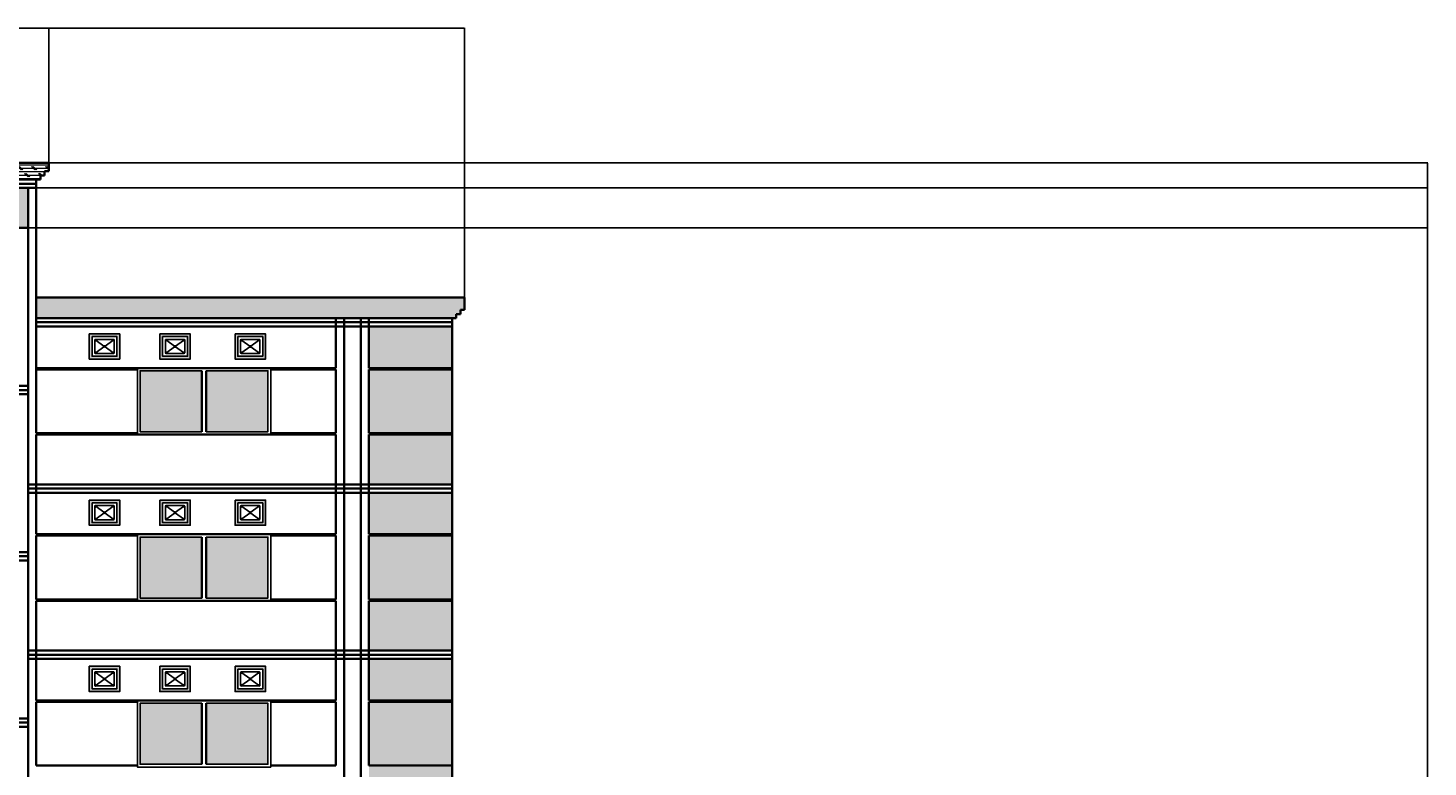
# Model space of a CAD drawing. Units: inches. Extents: x -742 to 1386, y -64 to 951.
# Tile 8 of 8: x 376 to 1386, y 418 to 951. Entities that reach past the tile are written whole.
import ezdxf

# ---------------------------------------------------------------- set-up
doc = ezdxf.new("R2010")
doc.units = ezdxf.units.IN
doc.header["$MEASUREMENT"] = 0
for name, color, linetype, lineweight in [('A-ANNO-DIMS', 2, 'Continuous', 18), ('A-ELEV', 7, 'Continuous', 35), ('A-ELEV-PATT', 252, 'Continuous', 13), ('A-GLAZ', 4, 'Continuous', 25), ('A-WALL-PATT', 8, 'Continuous', 13)]:
    doc.layers.add(name, color=color, linetype=linetype, lineweight=lineweight)
doc.styles.get("Standard").update_dxf_attribs({"font": 'arial.ttf'})
doc.dimstyles.get("Standard").update_dxf_attribs({"dimtxt": 0.18, "dimasz": 0.18, "dimexe": 0.18, "dimexo": 0.0625, "dimgap": 0.09, "dimtad": 0, "dimtih": 1, "dimtoh": 1, "dimdec": 4, "dimzin": 0, "dimdsep": 46, "dimtxsty": 'Standard', "dimcen": 0.09, "dimadec": 0, "dimazin": 0, "dimtfac": 1, "dimtdec": 4, "dimtofl": 0, "dimtmove": 0, "dimatfit": 3, "dimfxl": 1, "dimtolj": 1, "dimtzin": 0, "dimarcsym": 0})

# ---------------------------------------------------------------- blocks, each defined once
blk = doc.blocks.new('VENT-WIN')
h = blk.add_hatch(color=256)
h.dxf.hatch_style = 1
h.paths.add_polyline_path([(11.5, 9.1, 1), (10.5, 9.1, 1)])
h.paths.add_polyline_path([(16.9, 13.7, 1), (18, 13.7, 1)])
h.paths.add_polyline_path([(18, 4.5, 1), (16.9, 4.5, 1)])
h.paths.add_polyline_path([(5, 4.5, 1), (4, 4.5, 1)])
h.paths.add_polyline_path([(4, 13.7, 1), (5, 13.7, 1)])
for p, q in [((5, 13.5), (10.6, 9.4)), ((11.4, 9.4), (17, 13.5)), ((5, 4.7), (10.6, 8.8)), ((11.4, 8.8), (17, 4.7))]:
    blk.add_line(p, q)
for points in [[(0, 18.2), (22, 18.2), (22, 0), (0, 0)], [(2, 16.2), (20, 16.2), (20, 2), (2, 2)]]:
    blk.add_lwpolyline(points, close=True)
for points in [[(4, 4.5), (4, 13.7)], [(4.5, 14.2), (17.5, 14.2)], [(18, 13.7), (18, 4.5)], [(17.5, 4), (4.5, 4)]]:
    blk.add_lwpolyline(points)
for centre in [(4.5, 13.7), (17.5, 13.7), (4.5, 4.5), (11, 9.1), (17.5, 4.5)]:
    blk.add_circle(centre, 0.519)
blk = doc.blocks.new('WIN-1000-2PANE')
blk.add_lwpolyline([(0, 48), (96.2, 48), (96.2, 0), (0, 0)], close=True)
for points in [[(46.6, 2), (2, 2), (2, 46), (46.6, 46)], [(49.6, 46), (94.2, 46), (94.2, 2), (49.6, 2)]]:
    blk.add_lwpolyline(points)
blk = doc.blocks.new('*D10')
at = {"layer": 'A-ANNO-DIMS', "color": 0, "lineweight": -2, "transparency": 16777216}
for p, q in [((-46.8, 756.8), (-46.8, 951.2)), ((-46.6, 951), (321.9, 951)), ((691, 951), (322.5, 951)), ((691.2, 756.8), (691.2, 951.2))]:
    blk.add_line(p, q, dxfattribs=at)
at = {"layer": 'A-ANNO-DIMS', "color": 0, "transparency": 16777216}
for points in [[(-46.6, 951.1), (-46.6, 951), (-46.8, 951)], [(691, 951.1), (691, 951), (691.2, 951)]]:
    blk.add_solid(points, dxfattribs=at)
at = {"layer": 'Defpoints', "color": 0, "transparency": 16777216}
for p in [(691.2, 951), (-46.8, 756.7), (691.2, 756.7)]:
    blk.add_point(p, dxfattribs=at)
at = {"layer": 'A-ANNO-DIMS', "color": 0, "transparency": 16777216, "insert": (322.2, 951), "char_height": 0.18, "attachment_point": 5}
blk.add_mtext('\\A1;738', dxfattribs=at)
blk = doc.blocks.new('*D11')
at = {"layer": 'A-ANNO-DIMS', "color": 0, "lineweight": -2, "transparency": 16777216}
for p, q in [((253.2, 853.8), (253.2, 951.2)), ((253.4, 951), (321.9, 951)), ((391, 951), (322.5, 951)), ((391.2, 853.8), (391.2, 951.2))]:
    blk.add_line(p, q, dxfattribs=at)
at = {"layer": 'A-ANNO-DIMS', "color": 0, "transparency": 16777216}
for points in [[(253.4, 951.1), (253.4, 951), (253.2, 951)], [(391, 951.1), (391, 951), (391.2, 951)]]:
    blk.add_solid(points, dxfattribs=at)
at = {"layer": 'Defpoints', "color": 0, "transparency": 16777216}
for p in [(391.2, 951), (253.2, 853.8), (391.2, 853.8)]:
    blk.add_point(p, dxfattribs=at)
at = {"layer": 'A-ANNO-DIMS', "color": 0, "transparency": 16777216, "insert": (322.2, 951), "char_height": 0.18, "attachment_point": 5}
blk.add_mtext('\\A1;138', dxfattribs=at)
blk = doc.blocks.new('*D39')
at = {"layer": 'A-ANNO-DIMS', "color": 0, "lineweight": -2, "transparency": 16777216}
for p, q in [((391.3, 853.8), (1386, 853.8)), ((1385.8, 853.6), (1385.8, 479.9)), ((1385.8, 105.9), (1385.8, 479.6)), ((682.3, 105.7), (1386, 105.7))]:
    blk.add_line(p, q, dxfattribs=at)
at = {"layer": 'A-ANNO-DIMS', "color": 0, "transparency": 16777216}
for points in [[(1385.8, 853.6), (1385.9, 853.6), (1385.8, 853.8)], [(1385.8, 105.9), (1385.9, 105.9), (1385.8, 105.7)]]:
    blk.add_solid(points, dxfattribs=at)
at = {"layer": 'Defpoints', "color": 0, "transparency": 16777216}
for p in [(391.2, 853.8), (682.2, 105.7), (1385.8, 105.7)]:
    blk.add_point(p, dxfattribs=at)
at = {"layer": 'A-ANNO-DIMS', "color": 0, "transparency": 16777216, "insert": (1385.8, 479.8), "char_height": 0.18, "attachment_point": 5}
blk.add_mtext('\\A1;748', dxfattribs=at)
blk = doc.blocks.new('*D57')
at = {"layer": 'A-ANNO-DIMS', "color": 0, "lineweight": -2, "transparency": 16777216}
for p, q in [((376.3, 835.8), (1386, 835.8)), ((1385.8, 835.6), (1385.8, 821.5)), ((1385.8, 807), (1385.8, 821.1)), ((346.8, 806.9), (1386, 806.9))]:
    blk.add_line(p, q, dxfattribs=at)
at = {"layer": 'A-ANNO-DIMS', "color": 0, "transparency": 16777216}
for points in [[(1385.8, 835.6), (1385.9, 835.6), (1385.8, 835.8)], [(1385.8, 807), (1385.9, 807), (1385.8, 806.9)]]:
    blk.add_solid(points, dxfattribs=at)
at = {"layer": 'Defpoints', "color": 0, "transparency": 16777216}
for p in [(376.2, 835.8), (1385.8, 835.8), (346.7, 806.9)]:
    blk.add_point(p, dxfattribs=at)
at = {"layer": 'A-ANNO-DIMS', "color": 0, "transparency": 16777216, "insert": (1385.8, 821.3), "char_height": 0.18, "attachment_point": 5}
blk.add_mtext('\\A1;28.925', dxfattribs=at)

msp = doc.modelspace()

# ---------------------------------------------------------------- hatches: boundary and pattern name
at = {"layer": 'A-ELEV-PATT'}
h = msp.add_hatch(color=256, dxfattribs=at)
h.dxf.hatch_style = 1
h.paths.add_polyline_path([(442.4136, 730.4496), (420.4263, 730.4496), (420.4263, 712.2254), (442.4136, 712.2254)])
h.paths.add_polyline_path([(440.4136, 714.2254), (422.4263, 714.2254), (422.4263, 728.4496), (440.4136, 728.4496)], flags=16)
h.paths.add_polyline_path([(493.3109, 730.4496), (471.3236, 730.4496), (471.3236, 712.2254), (493.3109, 712.2254)])
h.paths.add_polyline_path([(491.3109, 728.4496), (491.3109, 714.2254), (473.3236, 714.2254), (473.3236, 728.4496)], flags=16)
h.paths.add_polyline_path([(547.5617, 730.4496), (525.5743, 730.4496), (525.5743, 712.2254), (547.5617, 712.2254)])
h.paths.add_polyline_path([(545.5617, 728.4496), (545.5617, 714.2254), (527.5743, 714.2254), (527.5743, 728.4496)], flags=16)
h = msp.add_hatch(color=256, dxfattribs=at)
h.dxf.hatch_style = 1
h.set_gradient(color1=(0, 255, 255), name='CURVED')
h.paths.add_polyline_path([(139.7128, 703.7399), (95.1117, 703.7399), (95.1117, 659.7399), (139.7128, 659.7399)])
h.paths.add_polyline_path([(187.3139, 703.7399), (142.7128, 703.7399), (142.7128, 659.7399), (187.3139, 659.7399)])
h.paths.add_polyline_path([(501.7423, 703.7399), (457.1413, 703.7399), (457.1413, 659.7399), (501.7423, 659.7399)])
h.paths.add_polyline_path([(549.3434, 703.7399), (504.7423, 703.7399), (504.7423, 659.7399), (549.3434, 659.7399)])
h = msp.add_hatch(color=256, dxfattribs=at)
h.dxf.hatch_style = 1
h.paths.add_polyline_path([(442.4136, 610.4496), (420.4263, 610.4496), (420.4263, 592.2254), (442.4136, 592.2254)])
h.paths.add_polyline_path([(440.4136, 594.2254), (422.4263, 594.2254), (422.4263, 608.4496), (440.4136, 608.4496)], flags=16)
h.paths.add_polyline_path([(493.3109, 610.4496), (471.3236, 610.4496), (471.3236, 592.2254), (493.3109, 592.2254)])
h.paths.add_polyline_path([(491.3109, 608.4496), (491.3109, 594.2254), (473.3236, 594.2254), (473.3236, 608.4496)], flags=16)
h.paths.add_polyline_path([(547.5617, 610.4496), (525.5743, 610.4496), (525.5743, 592.2254), (547.5617, 592.2254)])
h.paths.add_polyline_path([(545.5617, 608.4496), (545.5617, 594.2254), (527.5743, 594.2254), (527.5743, 608.4496)], flags=16)
h = msp.add_hatch(color=256, dxfattribs=at)
h.dxf.hatch_style = 1
h.set_gradient(color1=(0, 255, 255), name='CURVED')
h.paths.add_polyline_path([(139.7128, 583.7399), (95.1117, 583.7399), (95.1117, 539.7399), (139.7128, 539.7399)])
h.paths.add_polyline_path([(187.3139, 583.7399), (142.7128, 583.7399), (142.7128, 539.7399), (187.3139, 539.7399)])
h.paths.add_polyline_path([(501.7423, 583.7399), (457.1413, 583.7399), (457.1413, 539.7399), (501.7423, 539.7399)])
h.paths.add_polyline_path([(549.3434, 583.7399), (504.7423, 583.7399), (504.7423, 539.7399), (549.3434, 539.7399)])
h = msp.add_hatch(color=256, dxfattribs=at)
h.dxf.hatch_style = 1
h.paths.add_polyline_path([(442.4136, 490.4496), (420.4263, 490.4496), (420.4263, 472.2254), (442.4136, 472.2254)])
h.paths.add_polyline_path([(440.4136, 474.2254), (422.4263, 474.2254), (422.4263, 488.4496), (440.4136, 488.4496)], flags=16)
h.paths.add_polyline_path([(493.3109, 490.4496), (471.3236, 490.4496), (471.3236, 472.2254), (493.3109, 472.2254)])
h.paths.add_polyline_path([(491.3109, 488.4496), (491.3109, 474.2254), (473.3236, 474.2254), (473.3236, 488.4496)], flags=16)
h.paths.add_polyline_path([(547.5617, 490.4496), (525.5743, 490.4496), (525.5743, 472.2254), (547.5617, 472.2254)])
h.paths.add_polyline_path([(545.5617, 488.4496), (545.5617, 474.2254), (527.5743, 474.2254), (527.5743, 488.4496)], flags=16)
h = msp.add_hatch(color=256, dxfattribs=at)
h.dxf.hatch_style = 1
h.set_gradient(color1=(0, 255, 255), name='CURVED')
h.paths.add_polyline_path([(139.7128, 463.7399), (95.1117, 463.7399), (95.1117, 419.7399), (139.7128, 419.7399)])
h.paths.add_polyline_path([(187.3139, 463.7399), (142.7128, 463.7399), (142.7128, 419.7399), (187.3139, 419.7399)])
h.paths.add_polyline_path([(501.7423, 463.7399), (457.1413, 463.7399), (457.1413, 419.7399), (501.7423, 419.7399)])
h.paths.add_polyline_path([(549.3434, 463.7399), (504.7423, 463.7399), (504.7423, 419.7399), (549.3434, 419.7399)])
at = {"layer": 'A-WALL-PATT', "transparency": 33554457}
h = msp.add_hatch(dxfattribs=at)
h.set_pattern_fill('CORK', color=256, scale=20)
h.set_pattern_definition([(0, (0, 0), (0, 2.5), []), (135, (1.25, -1.25), (-5, -5), [3.535534, -3.535534]), (135, (1.875, -1.25), (-5, -5), [3.535534, -3.535534]), (135, (2.5, -1.25), (-5, -5), [3.535534, -3.535534])])
h.paths.add_polyline_path([(382.2276, 841.7799), (385.2276, 841.7799), (385.2276, 844.7799), (388.2276, 844.7799), (388.2276, 847.7799), (391.2276, 847.7799), (391.2276, 853.7799), (253.2276, 853.7799), (253.2276, 847.7799), (256.2276, 847.7799), (256.2276, 844.7799), (259.2276, 844.7799), (259.2276, 841.7799), (262.2276, 841.7799)])
h = msp.add_hatch(dxfattribs=at)
h.set_pattern_fill('AR-B88', color=256)
h.paths.add_polyline_path([(22.2276, 224.7399), (-37.7724, 224.7399), (-37.7724, 178.7399), (22.2276, 178.7399)])
h.paths.add_polyline_path([(22.2276, 177.7399), (-37.7724, 177.7399), (-37.7724, 141.7399), (22.2276, 141.7399)])
h.paths.add_polyline_path([(22.2276, 255.7399), (-37.7724, 255.7399), (-37.7724, 225.7399), (22.2276, 225.7399)])
h.paths.add_polyline_path([(22.2276, 297.7399), (-37.7724, 297.7399), (-37.7724, 261.7399), (22.2276, 261.7399)])
h.paths.add_polyline_path([(22.2276, 344.7399), (-37.7724, 344.7399), (-37.7724, 298.7399), (22.2276, 298.7399)])
h.paths.add_polyline_path([(22.2276, 375.7399), (-37.7724, 375.7399), (-37.7724, 345.7399), (22.2276, 345.7399)])
h.paths.add_polyline_path([(22.2276, 417.7399), (-37.7724, 417.7399), (-37.7724, 381.7399), (22.2276, 381.7399)])
h.paths.add_polyline_path([(22.2276, 464.7399), (-37.7724, 464.7399), (-37.7724, 418.7399), (22.2276, 418.7399)])
h.paths.add_polyline_path([(22.2276, 495.7399), (-37.7724, 495.7399), (-37.7724, 465.7399), (22.2276, 465.7399)])
h.paths.add_polyline_path([(22.2276, 537.7399), (-37.7724, 537.7399), (-37.7724, 501.7399), (22.2276, 501.7399)])
h.paths.add_polyline_path([(22.2276, 584.7399), (-37.7724, 584.7399), (-37.7724, 538.7399), (22.2276, 538.7399)])
h.paths.add_polyline_path([(22.2276, 615.7399), (-37.7724, 615.7399), (-37.7724, 585.7399), (22.2276, 585.7399)])
h.paths.add_polyline_path([(22.2276, 657.7399), (-37.7724, 657.7399), (-37.7724, 621.7399), (22.2276, 621.7399)])
h.paths.add_polyline_path([(22.2276, 704.7399), (-37.7724, 704.7399), (-37.7724, 658.7399), (22.2276, 658.7399)])
h.paths.add_polyline_path([(22.2276, 735.7399), (-37.7724, 735.7399), (-37.7724, 705.7399), (22.2276, 705.7399)])
h.paths.add_polyline_path([(376.2276, 835.7799), (268.2276, 835.7799), (268.2276, 806.8548), (376.2276, 806.8548)])
h.paths.add_polyline_path([(682.2276, 735.7399), (622.2276, 735.7399), (622.2276, 705.7399), (682.2276, 705.7399)])
h.paths.add_polyline_path([(682.2276, 704.7399), (622.2276, 704.7399), (622.2276, 658.7399), (682.2276, 658.7399)])
h.paths.add_polyline_path([(682.2276, 657.7399), (622.2276, 657.7399), (622.2276, 621.7399), (682.2276, 621.7399)])
h.paths.add_polyline_path([(682.2276, 615.7399), (622.2276, 615.7399), (622.2276, 585.7399), (682.2276, 585.7399)])
h.paths.add_polyline_path([(682.2276, 584.7399), (622.2276, 584.7399), (622.2276, 538.7399), (682.2276, 538.7399)])
h.paths.add_polyline_path([(682.2276, 537.7399), (622.2276, 537.7399), (622.2276, 501.7399), (682.2276, 501.7399)])
h.paths.add_polyline_path([(682.2276, 495.7399), (622.2276, 495.7399), (622.2276, 465.7399), (682.2276, 465.7399)])
h.paths.add_polyline_path([(682.2276, 464.7399), (622.2276, 464.7399), (622.2276, 418.7399), (682.2276, 418.7399)])
h.paths.add_polyline_path([(682.2276, 417.7399), (622.2276, 417.7399), (622.2276, 381.7399), (682.2276, 381.7399)])
h.paths.add_polyline_path([(682.2276, 375.7399), (622.2276, 375.7399), (622.2276, 345.7399), (682.2276, 345.7399)])
h.paths.add_polyline_path([(682.2276, 344.7399), (622.2276, 344.7399), (622.2276, 298.7399), (682.2276, 298.7399)])
h.paths.add_polyline_path([(682.2276, 297.7399), (622.2276, 297.7399), (622.2276, 261.7399), (682.2276, 261.7399)])
h.paths.add_polyline_path([(682.2276, 255.7399), (622.2276, 255.7399), (622.2276, 225.7399), (682.2276, 225.7399)])
h.paths.add_polyline_path([(682.2276, 224.7399), (622.2276, 224.7399), (622.2276, 178.7399), (682.2276, 178.7399)])
h.paths.add_polyline_path([(682.2276, 177.7399), (622.2276, 177.7399), (622.2276, 141.7399), (682.2276, 141.7399)])
h = msp.add_hatch(dxfattribs=at)
h.set_pattern_fill('CORK', color=256, scale=30, angle=91)
h.set_pattern_definition([(91, (0, 0), (-3.749429, -0.065447), []), (226, (1.842, 1.907), (7.62975, -7.36796), [5.3033, -5.3033]), (226, (1.826, 2.845), (7.62975, -7.36796), [5.3033, -5.3033]), (226, (1.809, 3.782), (7.62975, -7.36796), [5.3033, -5.3033])])
h.paths.add_polyline_path([(262.2276, 756.7399), (-46.7724, 756.7399), (-46.7724, 753.7399), (-46.7724, 747.7399), (-43.7724, 747.7399), (-43.7724, 744.7399), (-40.7724, 744.7399), (-40.7724, 741.7399), (-37.7724, 741.7399), (262.2276, 741.7399)])
h.paths.add_polyline_path([(688.2276, 747.7399), (691.2276, 747.7399), (691.2276, 753.7399), (691.2276, 756.7399), (382.2276, 756.7399), (382.2276, 741.7399), (682.2276, 741.7399), (685.2276, 741.7399), (685.2276, 744.7399), (688.2276, 744.7399)])

# ---------------------------------------------------------------- linework, layer by layer
at = {"layer": 'A-ELEV'}
for p, q in [((253.2276, 853.7799), (391.2276, 853.7799)), ((391.2276, 847.7799), (391.2276, 853.7799)), ((382.2276, 841.7799), (262.2276, 841.7799)), ((382.2276, 838.7799), (262.2276, 838.7799)), ((382.2276, 835.7799), (382.2276, 841.7799)), ((382.2276, 841.7799), (385.2276, 841.7799)), ((385.2276, 841.7799), (385.2276, 844.7799)), ((385.2276, 844.7799), (388.2276, 844.7799)), ((388.2276, 844.7799), (388.2276, 847.7799)), ((388.2276, 847.7799), (391.2276, 847.7799)), ((382.2276, 835.7799), (262.2276, 835.7799)), ((376.2276, 105.7399), (376.2276, 835.7799)), ((382.2276, 704.7399), (382.2276, 835.7799)), ((268.2276, 806.8548), (376.2276, 806.8548)), ((691.2276, 756.7399), (382.2276, 756.7399)), ((688.2276, 744.7399), (688.2276, 747.7399)), ((688.2276, 747.7399), (691.2276, 747.7399)), ((691.2276, 753.7399), (691.2276, 756.7399)), ((691.2276, 747.7399), (691.2276, 753.7399)), ((382.2276, 741.7399), (682.2276, 741.7399)), ((382.2276, 738.7399), (682.2276, 738.7399)), ((598.2276, 705.7399), (598.2276, 741.7399)), ((604.2276, 141.7399), (604.2276, 741.7399)), ((616.2276, 141.7399), (616.2276, 741.7399)), ((622.2276, 705.7399), (622.2276, 741.7399)), ((682.2276, 141.7399), (682.2276, 741.7399)), ((682.2276, 741.7399), (685.2276, 741.7399)), ((685.2276, 741.7399), (685.2276, 744.7399)), ((685.2276, 744.7399), (688.2276, 744.7399)), ((382.2276, 735.7399), (682.2276, 735.7399)), ((598.2276, 705.7399), (382.2276, 705.7399)), ((455.1413, 704.7399), (382.2276, 704.7399)), ((382.2276, 658.7399), (382.2276, 704.7399)), ((501.7423, 703.7399), (501.7423, 659.7399)), ((504.7423, 703.7399), (504.7423, 659.7399)), ((598.2276, 704.7399), (551.3434, 704.7399)), ((598.2276, 658.7399), (598.2276, 704.7399)), ((682.2276, 705.7399), (622.2276, 705.7399)), ((682.2276, 704.7399), (622.2276, 704.7399)), ((622.2276, 658.7399), (622.2276, 704.7399)), ((376.2276, 692.8548), (268.2276, 692.8548)), ((376.2276, 689.8548), (268.2276, 689.8548)), ((376.2276, 686.8548), (268.2276, 686.8548)), ((455.1413, 658.7399), (382.2276, 658.7399)), ((598.2276, 657.7399), (382.2276, 657.7399)), ((382.2276, 585.7399), (382.2276, 657.7399)), ((598.2276, 658.7399), (551.3434, 658.7399)), ((598.2276, 585.7399), (598.2276, 657.7399)), ((682.2276, 658.7399), (622.2276, 658.7399)), ((682.2276, 657.7399), (622.2276, 657.7399)), ((622.2276, 585.7399), (622.2276, 657.7399)), ((376.2276, 621.7399), (682.2276, 621.7399)), ((376.2276, 618.7399), (682.2276, 618.7399)), ((376.2276, 615.7399), (682.2276, 615.7399)), ((598.2276, 585.7399), (382.2276, 585.7399)), ((455.1413, 584.7399), (382.2276, 584.7399)), ((382.2276, 538.7399), (382.2276, 584.7399)), ((501.7423, 583.7399), (501.7423, 539.7399)), ((504.7423, 583.7399), (504.7423, 539.7399)), ((598.2276, 584.7399), (551.3434, 584.7399)), ((598.2276, 538.7399), (598.2276, 584.7399)), ((682.2276, 585.7399), (622.2276, 585.7399)), ((682.2276, 584.7399), (622.2276, 584.7399)), ((622.2276, 538.7399), (622.2276, 584.7399)), ((376.2276, 572.8548), (268.2276, 572.8548)), ((376.2276, 569.8548), (268.2276, 569.8548)), ((376.2276, 566.8548), (268.2276, 566.8548)), ((455.1413, 538.7399), (382.2276, 538.7399)), ((598.2276, 537.7399), (382.2276, 537.7399)), ((382.2276, 465.7399), (382.2276, 537.7399)), ((598.2276, 538.7399), (551.3434, 538.7399)), ((598.2276, 465.7399), (598.2276, 537.7399)), ((682.2276, 538.7399), (622.2276, 538.7399)), ((682.2276, 537.7399), (622.2276, 537.7399)), ((622.2276, 465.7399), (622.2276, 537.7399)), ((376.2276, 501.7399), (682.2276, 501.7399)), ((376.2276, 498.7399), (682.2276, 498.7399)), ((376.2276, 495.7399), (682.2276, 495.7399)), ((598.2276, 465.7399), (382.2276, 465.7399)), ((455.1413, 464.7399), (382.2276, 464.7399)), ((382.2276, 418.7399), (382.2276, 464.7399)), ((598.2276, 464.7399), (551.3434, 464.7399)), ((598.2276, 418.7399), (598.2276, 464.7399)), ((682.2276, 465.7399), (622.2276, 465.7399)), ((682.2276, 464.7399), (622.2276, 464.7399)), ((622.2276, 418.7399), (622.2276, 464.7399)), ((501.7423, 463.7399), (501.7423, 419.7399)), ((504.7423, 463.7399), (504.7423, 419.7399)), ((376.2276, 452.8548), (268.2276, 452.8548)), ((376.2276, 449.8548), (268.2276, 449.8548)), ((376.2276, 446.8548), (268.2276, 446.8548)), ((455.1413, 418.7399), (382.2276, 418.7399)), ((598.2276, 418.7399), (551.3434, 418.7399)), ((682.2276, 418.7399), (622.2276, 418.7399))]:
    msp.add_line(p, q, dxfattribs=at)

# ---------------------------------------------------------------- block references
at = {"layer": 'A-GLAZ'}
for p in [(420.4267, 712.225), (471.324, 712.225), (525.5748, 712.225), (420.4267, 592.225), (471.324, 592.225), (525.5748, 592.225), (420.4267, 472.225), (471.324, 472.225), (525.5748, 472.225)]:
    msp.add_blockref('VENT-WIN', p, dxfattribs=at)
at = {"layer": 'A-GLAZ', "extrusion": (0, 0, -1), "zscale": -1}
for p in [(-551.3432, 657.74), (-551.3432, 537.74), (-551.3432, 417.74)]:
    msp.add_blockref('WIN-1000-2PANE', p, dxfattribs=at)

# ---------------------------------------------------------------- dimensions: what is measured, and where the dimension line sits
at = {"layer": 'A-ANNO-DIMS'}
for base, p1, p2, picture in [((691.2276, 951.0299), (-46.7724, 756.7399), (691.2276, 756.7399), '*D10'), ((391.2276, 951.0299), (253.2276, 853.7799), (391.2276, 853.7799), '*D11')]:
    dim = msp.add_linear_dim(base=base, p1=p1, p2=p2, dimstyle='Standard', override={"dimdec": 0, "dimlfac": 1, "dimrnd": 0, "dimzin": 0, "dimdsep": 46, "dimlunit": 2}, dxfattribs=at)
    dim.commit()
    dim.dimension.update_dxf_attribs({"geometry": picture, "text_midpoint": (322.2276, 951.0299)})
for base, p1, p2, override, picture, middle in [((1385.8262, 105.7399), (391.2276, 853.7799), (682.2276, 105.7399), {"dimdec": 0, "dimlfac": 1, "dimrnd": 0, "dimzin": 0, "dimdsep": 46, "dimlunit": 2}, '*D39', (1385.8262, 479.7599)), ((1385.8262, 835.7799), (346.6973, 806.8548), (376.2276, 835.7799), {"dimdec": 3, "dimlfac": 1, "dimrnd": 0, "dimzin": 0, "dimdsep": 46, "dimlunit": 2}, '*D57', (1385.8262, 821.3173))]:
    dim = msp.add_linear_dim(base=base, p1=p1, p2=p2, angle=90, dimstyle='Standard', override=override, dxfattribs=at)
    dim.commit()
    dim.dimension.update_dxf_attribs({"geometry": picture, "text_midpoint": middle})

doc.saveas('drawing.dxf')
